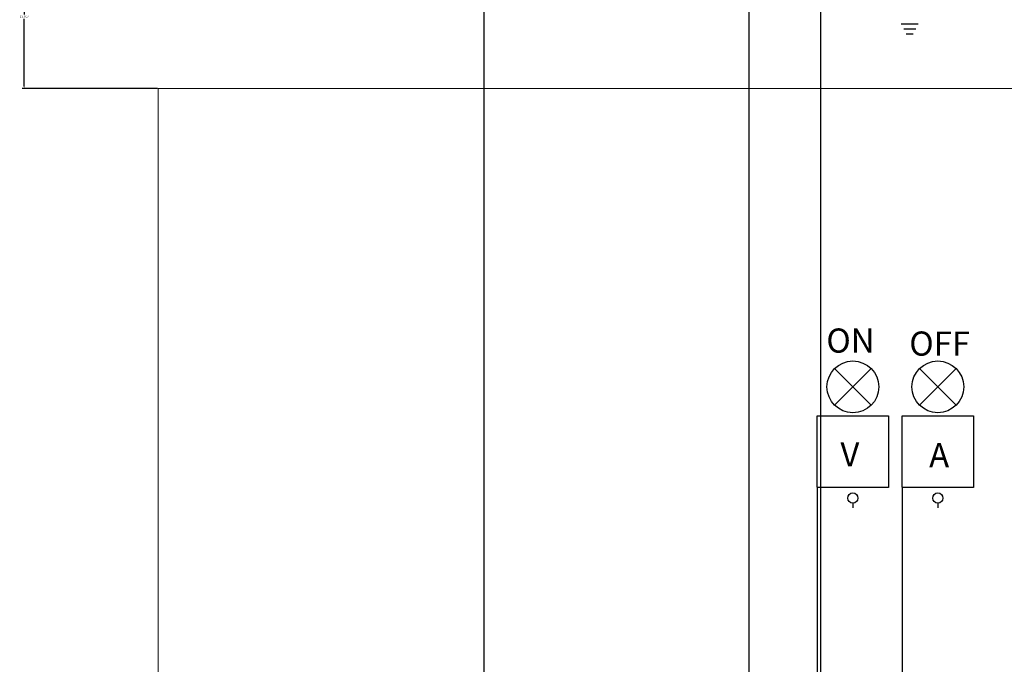
# Model space of a CAD drawing. Units: inches. Extents: x 412 to 584, y 208 to 437.
# Tile 5 of 28: x 412 to 494, y 262 to 315. Entities that reach past the tile are written whole.
import ezdxf

# ---------------------------------------------------------------- set-up
doc = ezdxf.new("R2010")
doc.units = ezdxf.units.IN
doc.header["$MEASUREMENT"] = 0
for name, color, linetype, lineweight in [('A-ANNO-DIMS', 2, 'Continuous', 18), ('E-ANNO-TEXT', 7, 'Continuous', 18), ('E-ENCL', 8, 'Continuous', 18), ('E-POWR-EQPM', 3, 'Continuous', 25)]:
    doc.layers.add(name, color=color, linetype=linetype, lineweight=lineweight)
doc.styles.get("Standard").update_dxf_attribs({"font": 'arial.ttf'})
doc.dimstyles.get("Standard").update_dxf_attribs({"dimtxt": 0.18, "dimasz": 0.18, "dimexe": 0.18, "dimexo": 0.0625, "dimgap": 0.09, "dimtad": 0, "dimtih": 1, "dimtoh": 1, "dimdec": 4, "dimzin": 0, "dimdsep": 46, "dimtxsty": 'Standard', "dimcen": 0.09, "dimadec": 0, "dimazin": 0, "dimtfac": 1, "dimtdec": 4, "dimtofl": 0, "dimtmove": 0, "dimatfit": 3, "dimfxl": 1, "dimtolj": 1, "dimtzin": 0, "dimarcsym": 0})

# ---------------------------------------------------------------- blocks, each defined once
blk = doc.blocks.new('*U1')
blk.add_line((0.758, -0.758), (-0.758, 0.758))
blk = doc.blocks.new('*U2')
at = {"color": 0, "linetype": 'ByBlock', "lineweight": -2, "transparency": 16777216}
blk.add_blockref('*U1', (78.828, 13.791), dxfattribs=at)
for p, rotation in [((80.344, 13.791), 269.9999999999999), ((78.828, 12.275), 89.99999999999996), ((80.344, 12.275), 180)]:
    blk.add_blockref('*U1', p, dxfattribs=dict(at, rotation=rotation))
blk = doc.blocks.new('INDICATOR-LAMP')
blk.add_circle((2.145, 2.145), 2.145)
at = {"rotation": 90.00000000000003}
blk.add_blockref('*U2', (15.178, -77.441), dxfattribs=at)
blk = doc.blocks.new('METER-VA')
blk.add_line((2.966, 0.398), (2.966, 0))
blk.add_lwpolyline([(0, 7.63), (5.932, 7.63), (5.932, 1.698), (0, 1.698)], close=True)
blk.add_circle((2.966, 0.821), 0.423)
blk = doc.blocks.new('*D26')
at = {"layer": 'A-ANNO-DIMS', "color": 0, "lineweight": -2, "transparency": 16777216}
for p, q in [((499.225, 321.294), (412.276, 321.294)), ((412.456, 321.114), (412.456, 315.518)), ((412.456, 309.557), (412.456, 315.154)), ((423.494, 309.377), (412.276, 309.377))]:
    blk.add_line(p, q, dxfattribs=at)
at = {"layer": 'A-ANNO-DIMS', "color": 0, "transparency": 16777216}
for points in [[(412.426, 321.114), (412.486, 321.114), (412.456, 321.294)], [(412.426, 309.557), (412.486, 309.557), (412.456, 309.377)]]:
    blk.add_solid(points, dxfattribs=at)
at = {"layer": 'Defpoints', "color": 0, "transparency": 16777216}
for p in [(499.288, 321.294), (412.456, 309.377), (423.556, 309.377)]:
    blk.add_point(p, dxfattribs=at)
at = {"layer": 'A-ANNO-DIMS', "color": 0, "transparency": 16777216, "insert": (412.456, 315.336), "char_height": 0.18, "attachment_point": 5}
blk.add_mtext('\\A1;11.917', dxfattribs=at)
blk = doc.blocks.new('*D28')
at = {"layer": 'A-ANNO-DIMS', "color": 0, "lineweight": -2, "transparency": 16777216}
for p, q in [((450.562, 256.635), (450.562, 437.465)), ((450.742, 437.285), (502.724, 437.285)), ((555.616, 437.285), (503.634, 437.285)), ((555.796, 256.635), (555.796, 437.465))]:
    blk.add_line(p, q, dxfattribs=at)
at = {"layer": 'A-ANNO-DIMS', "color": 0, "transparency": 16777216}
for points in [[(450.742, 437.315), (450.742, 437.255), (450.562, 437.285)], [(555.616, 437.315), (555.616, 437.255), (555.796, 437.285)]]:
    blk.add_solid(points, dxfattribs=at)
at = {"layer": 'Defpoints', "color": 0, "transparency": 16777216}
for p in [(555.796, 437.285), (450.562, 256.573), (555.796, 256.573)]:
    blk.add_point(p, dxfattribs=at)
at = {"layer": 'A-ANNO-DIMS', "color": 0, "transparency": 16777216, "insert": (503.179, 437.285), "char_height": 0.18, "attachment_point": 5}
blk.add_mtext('\\A1;105.23', dxfattribs=at)
blk = doc.blocks.new('*D33')
at = {"layer": 'A-ANNO-DIMS', "color": 0, "lineweight": -2, "transparency": 16777216}
for p, q in [((472.49, 363.226), (472.49, 208.233)), ((478.422, 363.226), (478.422, 208.233)), ((472.67, 208.413), (475.064, 208.413)), ((478.242, 208.413), (475.849, 208.413))]:
    blk.add_line(p, q, dxfattribs=at)
at = {"layer": 'A-ANNO-DIMS', "color": 0, "transparency": 16777216}
for points in [[(472.67, 208.443), (472.67, 208.383), (472.49, 208.413)], [(478.242, 208.443), (478.242, 208.383), (478.422, 208.413)]]:
    blk.add_solid(points, dxfattribs=at)
at = {"layer": 'Defpoints', "color": 0, "transparency": 16777216}
for p in [(472.49, 363.289), (478.422, 363.289), (478.422, 208.413)]:
    blk.add_point(p, dxfattribs=at)
at = {"layer": 'A-ANNO-DIMS', "color": 0, "transparency": 16777216, "insert": (475.456, 208.413), "char_height": 0.18, "attachment_point": 5}
blk.add_mtext('\\A1;5.932', dxfattribs=at)
blk = doc.blocks.new('*D34')
at = {"layer": 'A-ANNO-DIMS', "color": 0, "lineweight": -2, "transparency": 16777216}
for p, q in [((478.144, 276.254), (478.144, 208.233)), ((485.182, 276.254), (485.182, 208.233)), ((478.324, 208.413), (481.27, 208.413)), ((485.002, 208.413), (482.056, 208.413))]:
    blk.add_line(p, q, dxfattribs=at)
at = {"layer": 'A-ANNO-DIMS', "color": 0, "transparency": 16777216}
for points in [[(478.324, 208.443), (478.324, 208.383), (478.144, 208.413)], [(485.002, 208.443), (485.002, 208.383), (485.182, 208.413)]]:
    blk.add_solid(points, dxfattribs=at)
at = {"layer": 'Defpoints', "color": 0, "transparency": 16777216}
for p in [(478.144, 276.317), (485.182, 276.317), (485.182, 208.413)]:
    blk.add_point(p, dxfattribs=at)
at = {"layer": 'A-ANNO-DIMS', "color": 0, "transparency": 16777216, "insert": (481.663, 208.413), "char_height": 0.18, "attachment_point": 5}
blk.add_mtext('\\A1;7.038', dxfattribs=at)

msp = doc.modelspace()

# ---------------------------------------------------------------- linework, layer by layer
at = {"layer": 'E-ENCL'}
msp.add_lwpolyline([(423.5562, 309.3773), (572.3937, 309.3773), (572.3937, 225.5881), (423.5562, 225.5881)], close=True, dxfattribs=at)
at = {"layer": 'E-POWR-EQPM'}
for p, q in [((485.1249, 314.7377), (486.5265, 314.7377)), ((485.3298, 314.3279), (486.3216, 314.3279)), ((485.5347, 313.9182), (486.1168, 313.9182))]:
    msp.add_line(p, q, dxfattribs=at)

# ---------------------------------------------------------------- block references
for p, rotation in [((478.9652, 286.7965), 269.9999999999978), ((486.0032, 286.7965), 269.9999999999989)]:
    msp.add_blockref('INDICATOR-LAMP', p, dxfattribs=dict(at, rotation=rotation))
for p in [(478.1434, 274.6189), (485.1814, 274.6189)]:
    msp.add_blockref('METER-VA', p, dxfattribs=at)

# ---------------------------------------------------------------- texts
at = {"layer": 'E-ANNO-TEXT', "char_height": 2, "attachment_point": 1}
for s, insert in [('\\pxqc;ON', (474.0947, 289.4891)), ('\\pxqc;OFF', (481.4855, 289.2387)), ('\\pxqc;V', (474.0443, 280.0606)), ('\\pxqc;A', (481.4402, 279.9874))]:
    msp.add_mtext_dynamic_manual_height_columns(s, width=13.633448, gutter_width=1, heights=[2.9648], dxfattribs=dict(at, insert=insert))

# ---------------------------------------------------------------- dimensions: what is measured, and where the dimension line sits
at = {"layer": 'A-ANNO-DIMS'}
for base, p1, p2, override, picture, middle in [((555.7959, 437.2847), (450.562, 256.5729), (555.7959, 256.5729), {"dimdec": 2, "dimlfac": 1, "dimrnd": 0, "dimzin": 0, "dimdsep": 46, "dimlunit": 2}, '*D28', (503.1789, 437.2847)), ((478.4225, 208.4133), (472.4903, 363.2888), (478.4225, 363.2888), {"dimdec": 3, "dimlfac": 1, "dimrnd": 0, "dimzin": 0, "dimdsep": 46, "dimlunit": 2}, '*D33', (475.4564, 208.4133)), ((485.1817, 208.4133), (478.1437, 276.3167), (485.1817, 276.3167), {"dimdec": 3, "dimlfac": 1, "dimrnd": 0, "dimzin": 0, "dimdsep": 46, "dimlunit": 2}, '*D34', (481.6627, 208.4133))]:
    dim = msp.add_linear_dim(base=base, p1=p1, p2=p2, dimstyle='Standard', override=override, dxfattribs=at)
    dim.commit()
    dim.dimension.update_dxf_attribs({"geometry": picture, "text_midpoint": middle})
dim = msp.add_linear_dim(base=(412.4562, 309.3773), p1=(499.2878, 321.2941), p2=(423.5562, 309.3773), angle=90, dimstyle='Standard', override={"dimdec": 3, "dimlfac": 1, "dimrnd": 0, "dimzin": 0, "dimdsep": 46, "dimlunit": 2}, dxfattribs=at)
dim.commit()
dim.dimension.update_dxf_attribs({"geometry": '*D26', "text_midpoint": (412.4562, 315.3357)})

doc.saveas('drawing.dxf')
